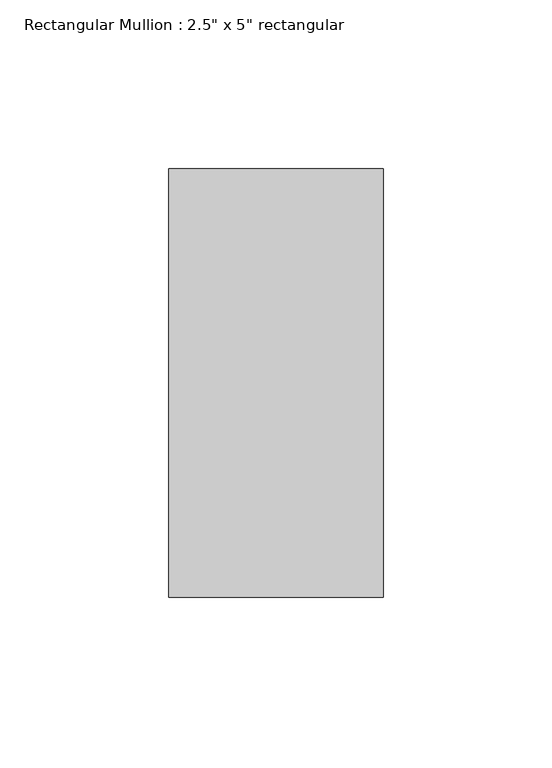
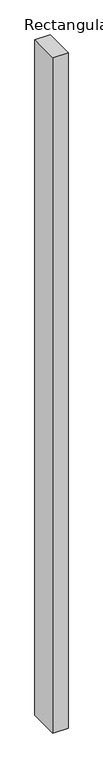
"""IFC4 building model written with IfcOpenShell, lengths in millimetres: member geometry."""

from ifc_helpers import new_model, si_unit, frame, origin, place, context, project, spatial, polyline, outline, extrude, source, transform, mapped, element, save


def member_19d0a4ec(model_context):
    return source(origin(), model_context, "Body", "SweptSolid", [
        extrude(outline(polyline([(31.75, 63.5), (31.75, -63.5), (-31.75, -63.5), (-31.75, 63.5), (31.75, 63.5)])), frame((0.0, 0.0, -2952.7500003), z_axis=(0.0, 0.0, 1.0), x_axis=(1.0, 0.0, 0.0)), (0.0, 0.0, 1.0), 2952.7500003),
    ])


if __name__ == "__main__":
    model = new_model("IFC4")
    model_context = context("Model", 3, world=origin())
    ifc_project = project(units=[si_unit("LENGTHUNIT", "METRE", prefix="MILLI")], contexts=[model_context])
    site = spatial("IfcSite", under=ifc_project)
    building = spatial("IfcBuilding", under=site)
    placement = place(None, origin())
    member_shape = member_19d0a4ec(model_context)
    element("IfcMember", 1, ObjectType="Rectangular Mullion : 2.5\" x 5\" rectangular", at=placement, inside=building, context=model_context, shape_type="MappedRepresentation", body=[
        mapped(member_shape, transform((0.0, 0.0, 0.0), x_axis=(1.0, 0.0, 0.0), y_axis=(0.0, 1.0, 0.0), z_axis=(0.0, 0.0, 1.0))),
    ])
    save(model, "model.ifc")

# Revit data of these elements
# Type "Rectangular Mullion : 2.5\" x 5\" rectangular"
#   built-in parameter 1007304 = 0.416667 (stored number, unit not read)
#   built-in parameter 1007301 = 0.104167 (stored number, unit not read)
#   built-in parameter 1007300 = 0.104167 (stored number, unit not read)
# Element 1 (IfcMember, "Rectangular Mullion : 2.5\" x 5\" rectangular")
#   Materials on its faces: "Aluminum"
# Materials
#   "Aluminum": class "Metal", colour RGB 247 247 247, transparency 0, Description = "Aluminum 6061", Cost = 0
